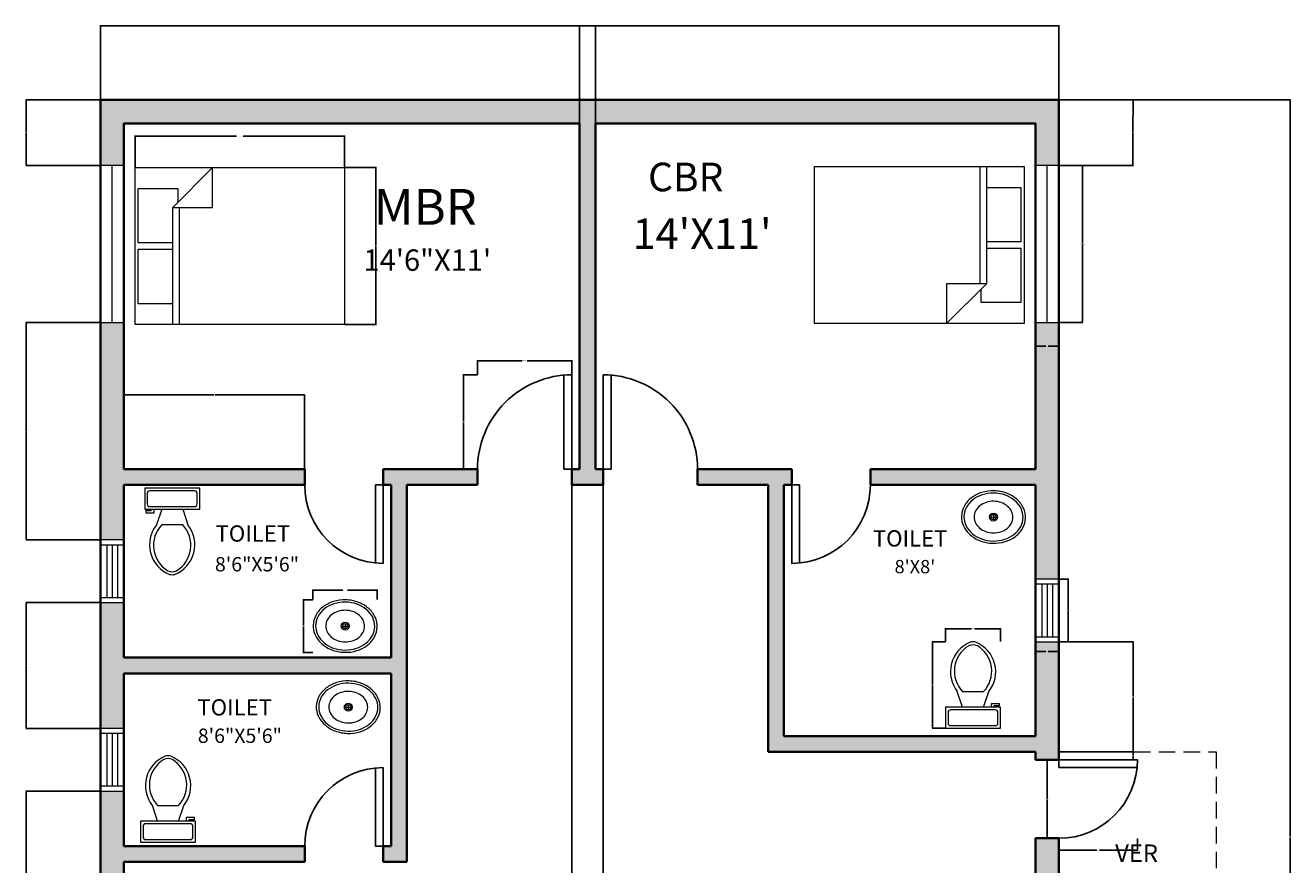
# Model space of a CAD drawing. Units: inches. Extents: x 60 to 543, y 115 to 735.
# Tile 2 of 2: x 60 to 543, y 415 to 735. Entities that reach past the tile are written whole.
import ezdxf

# ---------------------------------------------------------------- set-up
doc = ezdxf.new("R2010")
doc.units = ezdxf.units.IN
doc.linetypes.add('DASHED2', pattern=[9.525, 6.35, -3.175])
for name, color, linetype, lineweight in [('A-ANNO-DIMS', 2, 'Continuous', 18), ('A-AREA-IDEN', 7, 'Continuous', 18), ('A-DOOR', 4, 'Continuous', 25), ('A-FLOR-FIXT', 8, 'Continuous', 18), ('A-FLOR-OVHD', 8, 'DASHED2', 18), ('A-FURN', 8, 'Continuous', 18), ('A-GLAZ', 3, 'Continuous', 18), ('A-WALL', 7, 'Continuous', 35)]:
    doc.layers.add(name, color=color, linetype=linetype, lineweight=lineweight)
doc.layers.add('A-WALL-PATT', color=18, linetype='Continuous', lineweight=13, true_color=0x000000)
doc.styles.get("Standard").update_dxf_attribs({"font": 'arial.ttf'})
doc.dimstyles.get("Standard").update_dxf_attribs({"dimtxt": 0.18, "dimasz": 0.18, "dimexe": 0.18, "dimexo": 0.0625, "dimgap": 0.09, "dimtad": 0, "dimtih": 1, "dimtoh": 1, "dimdec": 4, "dimzin": 0, "dimdsep": 46, "dimtxsty": 'Standard', "dimcen": 0.09, "dimadec": 0, "dimazin": 0, "dimtfac": 1, "dimtdec": 4, "dimtofl": 0, "dimtmove": 0, "dimatfit": 3, "dimfxl": 1, "dimtolj": 1, "dimtzin": 0, "dimarcsym": 0})

# ---------------------------------------------------------------- blocks, each defined once
blk = doc.blocks.new('Bed - Queen')
for p, q in [((0, -80.00003), (0, 0)), ((0, 0), (59.99999, 0)), ((59.99999, 0), (59.99999, -80.00003)), ((7.99999, -1.2), (28.79998, -1.2)), ((7.99999, -14.4), (7.99999, -1.2)), ((28.79998, -1.2), (28.79998, -14.4)), ((31.19999, -1.2), (51.99999, -1.2)), ((31.19999, -14.4), (31.19999, -1.2)), ((51.99999, -1.2), (51.99999, -16.4)), ((0, -14.4), (44.8, -14.4)), ((59.99999, -29.6), (44.8, -14.4)), ((44.8, -14.4), (44.8, -29.6)), ((44.8, -16.8), (0, -16.8)), ((51.99999, -16.4), (46.79936, -16.4)), ((44.8, -29.6), (59.99999, -29.6)), ((59.99999, -80.00003), (0, -80.00003))]:
    blk.add_line(p, q)
blk = doc.blocks.new('Toilet - top')
for p, q in [((9.5, -6), (9.5, -2)), ((-10, -8.5), (-8, -8.5)), ((-10, -9.5), (-10, -8.5)), ((-7, -9.5), (-10, -9.5)), ((-8, -8.5), (-8, -8)), ((-7, -8), (-7, -9.5)), ((-4, -8), (-6, -14)), ((4, -8), (6, -14)), ((4, -14), (-4, -14))]:
    blk.add_line(p, q)
blk.add_lwpolyline([(10.5, -8), (10.5, 0), (-10.5, 0), (-10.5, -8)], close=True)
for points in [[(-9.5, -2), (-9.5, -6)], [(8.5, -1), (-8.5, -1)], [(-8.5, -7), (8.5, -7)]]:
    blk.add_lwpolyline(points)
for centre, radius, start, end in [((-8.62, -1.88), 0.884, 81.8699, 188.1301), ((8.62, -1.88), 0.884, 351.8699, 98.1301), ((-8.62, -6.12), 0.884, 171.8699, 278.1301), ((8.62, -6.12), 0.884, 261.8699, 8.1301), ((3.52, -21.58), 12.17, 141.4691, 247.9714), ((4.2, -21.82), 11.33, 136.3677, 238.9468), ((-3.52, -21.58), 12.17, 292.0284, 38.5307), ((-4.2, -21.82), 11.33, 301.053, 43.6321), ((0, -27.88), 4, 245.7318, 294.2682), ((0, -29), 4, 254.8605, 285.1395)]:
    blk.add_arc(centre, radius, start, end)
blk = doc.blocks.new('Sink - Oval top')
for p, q in [((-1, 0), (1, 0)), ((0, 1), (0, -1))]:
    blk.add_line(p, q)
for points in [[(-12.23, 0.39, 0.117634), (-11.46, -3.36, 0.104469), (-8.88, -6.8, 0.090016), (-5.08, -9.07, 0.08192), (-0.32, -10.02, 0.08192), (4.49, -9.38, 0.090016), (8.42, -7.36, 0.104469), (11.22, -4.09, 0.117634), (12.23, -0.39, 0.117634), (11.46, 3.36, 0.104469), (8.88, 6.8, 0.090016), (5.08, 9.07, 0.08192), (0.32, 10.02, 0.08192), (-4.49, 9.38, 0.090016), (-8.42, 7.36, 0.104469), (-11.22, 4.09, 0.117634)], [(-11.29, 0.16, 0.118622), (-10.52, -3.25, 0.104678), (-8.07, -6.36, 0.089562), (-4.54, -8.37, 0.081185), (-0.13, -9.15, 0.081185), (4.3, -8.49, 0.089562), (7.89, -6.58, 0.104678), (10.42, -3.55, 0.118622), (11.29, -0.16, 0.118622), (10.52, 3.25, 0.104678), (8.07, 6.36, 0.089562), (4.54, 8.37, 0.081185), (0.13, 9.15, 0.081185), (-4.3, 8.49, 0.089562), (-7.89, 6.58, 0.104678), (-10.42, 3.55, 0.118622)], [(-7.42, 0.08, 0.118283), (-6.91, -2.17, 0.104607), (-5.29, -4.21, 0.089718), (-2.97, -5.53, 0.081436), (-0.07, -6.04, 0.081436), (2.84, -5.59, 0.089718), (5.2, -4.33, 0.104607), (6.86, -2.32, 0.118283), (7.42, -0.08, 0.118283), (6.91, 2.17, 0.104607), (5.29, 4.21, 0.089718), (2.97, 5.53, 0.081436), (0.07, 6.04, 0.081436), (-2.84, 5.59, 0.089718), (-5.2, 4.33, 0.104607), (-6.86, 2.32, 0.118283)]]:
    blk.add_lwpolyline(points, format="xyb", close=True)
for radius in [1.5, 1]:
    blk.add_circle((0, 0), radius)
blk = doc.blocks.new('DOOR-SWING-36IN')
for p, q in [((0, 0), (0, 36)), ((0, 36), (3, 36)), ((3, 0), (3, 36))]:
    blk.add_line(p, q)
blk.add_arc((0, 36), 36, 270, 0)
blk = doc.blocks.new('DOOR-SWING-30IN')
for p, q in [((30, 30), (27, 30)), ((27, 0), (27, 30)), ((30, 0), (30, 30))]:
    blk.add_line(p, q)
blk.add_arc((30, 30), 30, 180, 270)
blk = doc.blocks.new('WINDOW-60IN')
for p, q in [((9, 60), (0, 60)), ((0, 60), (0, 0)), ((4.5, 0), (4.5, 60)), ((9, 0), (9, 60)), ((0, 0), (9, 0))]:
    blk.add_line(p, q)
blk = doc.blocks.new('BATH-VENT-24IN')
for p, q in [((0, 24), (0, 0)), ((9, 24), (0, 24)), ((9, 22), (0, 22)), ((2.5, 22), (2.5, 2)), ((4.5, 22), (4.5, 2)), ((6.5, 22), (6.5, 2)), ((9, 0), (9, 24)), ((0, 2), (9, 2)), ((0, 0), (9, 0))]:
    blk.add_line(p, q)
blk = doc.blocks.new('*D13')
at = {"layer": 'A-ANNO-DIMS', "color": 0, "lineweight": -2, "transparency": 16777216}
for p, q in [((454.43, 681.94), (463.55, 681.94)), ((463.37, 681.76), (463.37, 652.13)), ((463.37, 622.12), (463.37, 651.76)), ((454.43, 621.94), (463.55, 621.94))]:
    blk.add_line(p, q, dxfattribs=at)
at = {"layer": 'A-ANNO-DIMS', "color": 0, "transparency": 16777216}
for points in [[(463.34, 681.76), (463.4, 681.76), (463.37, 681.94)], [(463.34, 622.12), (463.4, 622.12), (463.37, 621.94)]]:
    blk.add_solid(points, dxfattribs=at)
at = {"layer": 'Defpoints', "color": 0, "transparency": 16777216}
for p in [(454.37, 681.94), (463.37, 681.94), (454.37, 621.94)]:
    blk.add_point(p, dxfattribs=at)
at = {"layer": 'A-ANNO-DIMS', "color": 0, "transparency": 16777216, "insert": (463.37, 651.94), "char_height": 0.18, "attachment_point": 5}
blk.add_mtext('\\A1;WINDOW 60 TYP.', dxfattribs=at)
blk = doc.blocks.new('*D14')
at = {"layer": 'A-ANNO-DIMS', "color": 0, "lineweight": -2, "transparency": 16777216}
for p, q in [((445.37, 621.88), (445.37, 612.76)), ((454.37, 621.88), (454.37, 612.76)), ((445.55, 612.94), (449.41, 612.94)), ((454.19, 612.94), (450.33, 612.94))]:
    blk.add_line(p, q, dxfattribs=at)
at = {"layer": 'A-ANNO-DIMS', "color": 0, "transparency": 16777216}
for points in [[(445.55, 612.97), (445.55, 612.91), (445.37, 612.94)], [(454.19, 612.97), (454.19, 612.91), (454.37, 612.94)]]:
    blk.add_solid(points, dxfattribs=at)
at = {"layer": 'Defpoints', "color": 0, "transparency": 16777216}
for p in [(445.37, 621.94), (454.37, 621.94), (454.37, 612.94)]:
    blk.add_point(p, dxfattribs=at)
at = {"layer": 'A-ANNO-DIMS', "color": 0, "transparency": 16777216, "insert": (449.87, 612.94), "char_height": 0.18, "attachment_point": 5}
blk.add_mtext('\\A1;9 TYP.', dxfattribs=at)
blk = doc.blocks.new('*D15')
at = {"layer": 'A-ANNO-DIMS', "color": 0, "lineweight": -2, "transparency": 16777216}
for p, q in [((454.33, 454.97), (449.71, 454.97)), ((449.89, 454.79), (449.89, 440.15)), ((449.89, 425.15), (449.89, 439.79)), ((454.33, 424.97), (449.71, 424.97))]:
    blk.add_line(p, q, dxfattribs=at)
at = {"layer": 'A-ANNO-DIMS', "color": 0, "transparency": 16777216}
for points in [[(449.86, 454.79), (449.92, 454.79), (449.89, 454.97)], [(449.86, 425.15), (449.92, 425.15), (449.89, 424.97)]]:
    blk.add_solid(points, dxfattribs=at)
at = {"layer": 'Defpoints', "color": 0, "transparency": 16777216}
for p in [(449.89, 454.97), (454.39, 454.97), (454.39, 424.97)]:
    blk.add_point(p, dxfattribs=at)
at = {"layer": 'A-ANNO-DIMS', "color": 0, "transparency": 16777216, "insert": (449.89, 439.97), "char_height": 0.18, "attachment_point": 5}
blk.add_mtext('\\A1;DOOR 30 TYP.', dxfattribs=at)
blk = doc.blocks.new('*D16')
at = {"layer": 'A-ANNO-DIMS', "color": 0, "lineweight": -2, "transparency": 16777216}
for p, q in [((454.39, 424.91), (454.39, 420.29)), ((454.57, 420.47), (468.87, 420.47)), ((484.21, 420.47), (469.92, 420.47)), ((484.39, 424.91), (484.39, 420.29))]:
    blk.add_line(p, q, dxfattribs=at)
at = {"layer": 'A-ANNO-DIMS', "color": 0, "transparency": 16777216}
for points in [[(454.57, 420.5), (454.57, 420.44), (454.39, 420.47)], [(484.21, 420.5), (484.21, 420.44), (484.39, 420.47)]]:
    blk.add_solid(points, dxfattribs=at)
at = {"layer": 'Defpoints', "color": 0, "transparency": 16777216}
for p in [(454.39, 424.97), (454.39, 420.47), (484.39, 424.97)]:
    blk.add_point(p, dxfattribs=at)
at = {"layer": 'A-ANNO-DIMS', "color": 0, "transparency": 16777216, "insert": (469.39, 420.47), "char_height": 0.18, "attachment_point": 5}
blk.add_mtext('\\A1;30 TYP.', dxfattribs=at)
blk = doc.blocks.new('*D17')
at = {"layer": 'A-ANNO-DIMS', "color": 0, "lineweight": -2, "transparency": 16777216}
for p, q in [((411.04, 500.05), (405.97, 500.05)), ((406.15, 499.87), (406.15, 483.71)), ((406.15, 467.18), (406.15, 483.34)), ((411.04, 467), (405.97, 467))]:
    blk.add_line(p, q, dxfattribs=at)
at = {"layer": 'A-ANNO-DIMS', "color": 0, "transparency": 16777216}
for points in [[(406.12, 499.87), (406.18, 499.87), (406.15, 500.05)], [(406.12, 467.18), (406.18, 467.18), (406.15, 467)]]:
    blk.add_solid(points, dxfattribs=at)
at = {"layer": 'Defpoints', "color": 0, "transparency": 16777216}
for p in [(411.1, 500.05), (406.15, 467), (411.1, 467)]:
    blk.add_point(p, dxfattribs=at)
at = {"layer": 'A-ANNO-DIMS', "color": 0, "transparency": 16777216, "insert": (406.15, 483.53), "char_height": 0.18, "attachment_point": 5}
blk.add_mtext('\\A1;WC 33 TYP.', dxfattribs=at)
blk = doc.blocks.new('*D18')
at = {"layer": 'A-ANNO-DIMS', "color": 0, "lineweight": -2, "transparency": 16777216}
for p, q in [((411.1, 500.11), (411.1, 505.19)), ((411.28, 505.01), (421.07, 505.01)), ((431.92, 505.01), (422.13, 505.01)), ((432.1, 500.11), (432.1, 505.19))]:
    blk.add_line(p, q, dxfattribs=at)
at = {"layer": 'A-ANNO-DIMS', "color": 0, "transparency": 16777216}
for points in [[(411.28, 505.04), (411.28, 504.98), (411.1, 505.01)], [(431.92, 505.04), (431.92, 504.98), (432.1, 505.01)]]:
    blk.add_solid(points, dxfattribs=at)
at = {"layer": 'Defpoints', "color": 0, "transparency": 16777216}
for p in [(411.1, 505.01), (411.1, 500.05), (432.1, 500.05)]:
    blk.add_point(p, dxfattribs=at)
at = {"layer": 'A-ANNO-DIMS', "color": 0, "transparency": 16777216, "insert": (421.6, 505.01), "char_height": 0.18, "attachment_point": 5}
blk.add_mtext('\\A1;21 TYP.', dxfattribs=at)
blk = doc.blocks.new('*D19')
at = {"layer": 'A-ANNO-DIMS', "color": 0, "lineweight": -2, "transparency": 16777216}
for p, q in [((169.57, 516.15), (169.57, 519.95)), ((169.75, 519.77), (180.91, 519.77)), ((193.94, 519.77), (182.78, 519.77)), ((194.12, 516.15), (194.12, 519.95))]:
    blk.add_line(p, q, dxfattribs=at)
at = {"layer": 'A-ANNO-DIMS', "color": 0, "transparency": 16777216}
for points in [[(169.75, 519.8), (169.75, 519.74), (169.57, 519.77)], [(193.94, 519.8), (193.94, 519.74), (194.12, 519.77)]]:
    blk.add_solid(points, dxfattribs=at)
at = {"layer": 'Defpoints', "color": 0, "transparency": 16777216}
for p in [(194.12, 519.77), (169.57, 516.09), (194.12, 516.09)]:
    blk.add_point(p, dxfattribs=at)
at = {"layer": 'A-ANNO-DIMS', "color": 0, "transparency": 16777216, "insert": (181.85, 519.77), "char_height": 0.18, "attachment_point": 5}
blk.add_mtext('\\A1;BASIN 25 TYP.', dxfattribs=at)
blk = doc.blocks.new('*D20')
at = {"layer": 'A-ANNO-DIMS', "color": 0, "lineweight": -2, "transparency": 16777216}
for p, q in [((169.51, 516.09), (165.71, 516.09)), ((165.89, 515.91), (165.89, 506.2)), ((165.89, 496.13), (165.89, 505.84)), ((169.51, 495.95), (165.71, 495.95))]:
    blk.add_line(p, q, dxfattribs=at)
at = {"layer": 'A-ANNO-DIMS', "color": 0, "transparency": 16777216}
for points in [[(165.86, 515.91), (165.92, 515.91), (165.89, 516.09)], [(165.86, 496.13), (165.92, 496.13), (165.89, 495.95)]]:
    blk.add_solid(points, dxfattribs=at)
at = {"layer": 'Defpoints', "color": 0, "transparency": 16777216}
for p in [(165.89, 516.09), (169.57, 516.09), (169.57, 495.95)]:
    blk.add_point(p, dxfattribs=at)
at = {"layer": 'A-ANNO-DIMS', "color": 0, "transparency": 16777216, "insert": (165.89, 506.02), "char_height": 0.18, "attachment_point": 5}
blk.add_mtext('\\A1;20 TYP.', dxfattribs=at)
blk = doc.blocks.new('*D21')
at = {"layer": 'A-ANNO-DIMS', "color": 0, "lineweight": -2, "transparency": 16777216}
for p, q in [((232.39, 602.03), (232.39, 607.55)), ((232.57, 607.37), (249.46, 607.37)), ((268.21, 607.37), (251.33, 607.37)), ((268.39, 602.03), (268.39, 607.55))]:
    blk.add_line(p, q, dxfattribs=at)
at = {"layer": 'A-ANNO-DIMS', "color": 0, "transparency": 16777216}
for points in [[(232.57, 607.4), (232.57, 607.34), (232.39, 607.37)], [(268.21, 607.4), (268.21, 607.34), (268.39, 607.37)]]:
    blk.add_solid(points, dxfattribs=at)
at = {"layer": 'Defpoints', "color": 0, "transparency": 16777216}
for p in [(232.39, 607.37), (232.39, 601.97), (268.39, 601.97)]:
    blk.add_point(p, dxfattribs=at)
at = {"layer": 'A-ANNO-DIMS', "color": 0, "transparency": 16777216, "insert": (250.39, 607.37), "char_height": 0.18, "attachment_point": 5}
blk.add_mtext('\\A1;DOOR 36 TYP.', dxfattribs=at)
blk = doc.blocks.new('*D22')
at = {"layer": 'A-ANNO-DIMS', "color": 0, "lineweight": -2, "transparency": 16777216}
for p, q in [((232.33, 601.97), (226.81, 601.97)), ((226.99, 601.79), (226.99, 584.15)), ((226.99, 566.15), (226.99, 583.79)), ((232.33, 565.97), (226.81, 565.97))]:
    blk.add_line(p, q, dxfattribs=at)
at = {"layer": 'A-ANNO-DIMS', "color": 0, "transparency": 16777216}
for points in [[(226.96, 601.79), (227.02, 601.79), (226.99, 601.97)], [(226.96, 566.15), (227.02, 566.15), (226.99, 565.97)]]:
    blk.add_solid(points, dxfattribs=at)
at = {"layer": 'Defpoints', "color": 0, "transparency": 16777216}
for p in [(232.39, 601.97), (226.99, 565.97), (232.39, 565.97)]:
    blk.add_point(p, dxfattribs=at)
at = {"layer": 'A-ANNO-DIMS', "color": 0, "transparency": 16777216, "insert": (226.99, 583.97), "char_height": 0.18, "attachment_point": 5}
blk.add_mtext('\\A1;36 TYP.', dxfattribs=at)
blk = doc.blocks.new('*D23')
at = {"layer": 'A-ANNO-DIMS', "color": 0, "lineweight": -2, "transparency": 16777216}
for p, q in [((454.46, 523.97), (458.17, 523.97)), ((457.99, 523.79), (457.99, 512.15)), ((457.99, 500.15), (457.99, 511.79)), ((454.46, 499.97), (458.17, 499.97))]:
    blk.add_line(p, q, dxfattribs=at)
at = {"layer": 'A-ANNO-DIMS', "color": 0, "transparency": 16777216}
for points in [[(457.96, 523.79), (458.02, 523.79), (457.99, 523.97)], [(457.96, 500.15), (458.02, 500.15), (457.99, 499.97)]]:
    blk.add_solid(points, dxfattribs=at)
at = {"layer": 'Defpoints', "color": 0, "transparency": 16777216}
for p in [(454.39, 523.97), (457.99, 523.97), (454.39, 499.97)]:
    blk.add_point(p, dxfattribs=at)
at = {"layer": 'A-ANNO-DIMS', "color": 0, "transparency": 16777216, "insert": (457.99, 511.97), "char_height": 0.18, "attachment_point": 5}
blk.add_mtext('\\A1;VENT 24 TYP.', dxfattribs=at)
blk = doc.blocks.new('*D24')
at = {"layer": 'A-ANNO-DIMS', "color": 0, "lineweight": -2, "transparency": 16777216}
for p, q in [((445.39, 499.91), (445.39, 496.19)), ((454.39, 499.91), (454.39, 496.19)), ((445.57, 496.37), (449.44, 496.37)), ((454.21, 496.37), (450.35, 496.37))]:
    blk.add_line(p, q, dxfattribs=at)
at = {"layer": 'A-ANNO-DIMS', "color": 0, "transparency": 16777216}
for points in [[(445.57, 496.4), (445.57, 496.34), (445.39, 496.37)], [(454.21, 496.4), (454.21, 496.34), (454.39, 496.37)]]:
    blk.add_solid(points, dxfattribs=at)
at = {"layer": 'Defpoints', "color": 0, "transparency": 16777216}
for p in [(445.39, 499.97), (454.39, 499.97), (454.39, 496.37)]:
    blk.add_point(p, dxfattribs=at)
at = {"layer": 'A-ANNO-DIMS', "color": 0, "transparency": 16777216, "insert": (449.89, 496.37), "char_height": 0.18, "attachment_point": 5}
blk.add_mtext('\\A1;9 TYP.', dxfattribs=at)
blk = doc.blocks.new('*D25')
at = {"layer": 'A-ANNO-DIMS', "color": 0, "lineweight": -2, "transparency": 16777216}
for p, q in [((101.61, 681.19), (101.61, 693.31)), ((101.79, 693.13), (140.31, 693.13)), ((181.43, 693.13), (142.91, 693.13)), ((181.61, 681.19), (181.61, 693.31))]:
    blk.add_line(p, q, dxfattribs=at)
at = {"layer": 'A-ANNO-DIMS', "color": 0, "transparency": 16777216}
for points in [[(101.79, 693.16), (101.79, 693.1), (101.61, 693.13)], [(181.43, 693.16), (181.43, 693.1), (181.61, 693.13)]]:
    blk.add_solid(points, dxfattribs=at)
at = {"layer": 'Defpoints', "color": 0, "transparency": 16777216}
for p in [(101.61, 693.13), (101.61, 681.13), (181.61, 681.13)]:
    blk.add_point(p, dxfattribs=at)
at = {"layer": 'A-ANNO-DIMS', "color": 0, "transparency": 16777216, "insert": (141.61, 693.13), "char_height": 0.18, "attachment_point": 5}
blk.add_mtext('\\A1;QUEEN BED 80 TYP.', dxfattribs=at)
blk = doc.blocks.new('*D26')
at = {"layer": 'A-ANNO-DIMS', "color": 0, "lineweight": -2, "transparency": 16777216}
for p, q in [((181.67, 681.13), (193.79, 681.13)), ((193.61, 680.95), (193.61, 651.31)), ((193.61, 621.31), (193.61, 650.95)), ((181.67, 621.13), (193.79, 621.13))]:
    blk.add_line(p, q, dxfattribs=at)
at = {"layer": 'A-ANNO-DIMS', "color": 0, "transparency": 16777216}
for points in [[(193.58, 680.95), (193.64, 680.95), (193.61, 681.13)], [(193.58, 621.31), (193.64, 621.31), (193.61, 621.13)]]:
    blk.add_solid(points, dxfattribs=at)
at = {"layer": 'Defpoints', "color": 0, "transparency": 16777216}
for p in [(181.61, 681.13), (193.61, 681.13), (181.61, 621.13)]:
    blk.add_point(p, dxfattribs=at)
at = {"layer": 'A-ANNO-DIMS', "color": 0, "transparency": 16777216, "insert": (193.61, 651.13), "char_height": 0.18, "attachment_point": 5}
blk.add_mtext('\\A1;60 TYP.', dxfattribs=at)
blk = doc.blocks.new('*D38')
at = {"layer": 'A-ANNO-DIMS', "color": 0, "lineweight": -2, "transparency": 16777216}
for p, q in [((454.46, 706.97), (542.87, 706.97)), ((542.69, 706.79), (542.69, 425.65)), ((542.69, 144.15), (542.69, 425.29)), ((454.46, 143.97), (542.87, 143.97))]:
    blk.add_line(p, q, dxfattribs=at)
at = {"layer": 'A-ANNO-DIMS', "color": 0, "transparency": 16777216}
for points in [[(542.66, 706.79), (542.72, 706.79), (542.69, 706.97)], [(542.66, 144.15), (542.72, 144.15), (542.69, 143.97)]]:
    blk.add_solid(points, dxfattribs=at)
at = {"layer": 'Defpoints', "color": 0, "transparency": 16777216}
for p in [(454.39, 706.97), (542.69, 706.97), (454.39, 143.97)]:
    blk.add_point(p, dxfattribs=at)
at = {"layer": 'A-ANNO-DIMS', "color": 0, "transparency": 16777216, "insert": (542.69, 425.47), "char_height": 0.18, "attachment_point": 5}
blk.add_mtext('\\A1;563', dxfattribs=at)
blk = doc.blocks.new('*D39')
at = {"layer": 'A-ANNO-DIMS', "color": 0, "lineweight": -2, "transparency": 16777216}
for p, q in [((88.39, 707.03), (88.39, 735.45)), ((88.57, 735.27), (271.1, 735.27)), ((454.21, 735.27), (271.68, 735.27)), ((454.39, 707.03), (454.39, 735.45))]:
    blk.add_line(p, q, dxfattribs=at)
at = {"layer": 'A-ANNO-DIMS', "color": 0, "transparency": 16777216}
for points in [[(88.57, 735.3), (88.57, 735.24), (88.39, 735.27)], [(454.21, 735.3), (454.21, 735.24), (454.39, 735.27)]]:
    blk.add_solid(points, dxfattribs=at)
at = {"layer": 'Defpoints', "color": 0, "transparency": 16777216}
for p in [(454.39, 735.27), (88.39, 706.97), (454.39, 706.97)]:
    blk.add_point(p, dxfattribs=at)
at = {"layer": 'A-ANNO-DIMS', "color": 0, "transparency": 16777216, "insert": (271.39, 735.27), "char_height": 0.18, "attachment_point": 5}
blk.add_mtext('\\A1;366', dxfattribs=at)
blk = doc.blocks.new('*D42')
at = {"layer": 'A-ANNO-DIMS', "color": 0, "lineweight": -2, "transparency": 16777216}
for p, q in [((88.33, 442.97), (59.91, 442.97)), ((60.09, 442.79), (60.09, 401.54)), ((60.09, 359.92), (60.09, 401.17)), ((88.33, 359.74), (59.91, 359.74))]:
    blk.add_line(p, q, dxfattribs=at)
at = {"layer": 'A-ANNO-DIMS', "color": 0, "transparency": 16777216}
for points in [[(60.06, 442.79), (60.12, 442.79), (60.09, 442.97)], [(60.06, 359.92), (60.12, 359.92), (60.09, 359.74)]]:
    blk.add_solid(points, dxfattribs=at)
at = {"layer": 'Defpoints', "color": 0, "transparency": 16777216}
for p in [(60.09, 442.97), (88.39, 442.97), (88.39, 359.74)]:
    blk.add_point(p, dxfattribs=at)
at = {"layer": 'A-ANNO-DIMS', "color": 0, "transparency": 16777216, "insert": (60.09, 401.35), "char_height": 0.18, "attachment_point": 5}
blk.add_mtext('\\A1;83.23', dxfattribs=at)
blk = doc.blocks.new('*D43')
at = {"layer": 'A-ANNO-DIMS', "color": 0, "lineweight": -2, "transparency": 16777216}
for p, q in [((88.33, 514.97), (59.91, 514.97)), ((60.09, 514.79), (60.09, 491.15)), ((60.09, 467.15), (60.09, 490.79)), ((88.33, 466.97), (59.91, 466.97))]:
    blk.add_line(p, q, dxfattribs=at)
at = {"layer": 'A-ANNO-DIMS', "color": 0, "transparency": 16777216}
for points in [[(60.06, 514.79), (60.12, 514.79), (60.09, 514.97)], [(60.06, 467.15), (60.12, 467.15), (60.09, 466.97)]]:
    blk.add_solid(points, dxfattribs=at)
at = {"layer": 'Defpoints', "color": 0, "transparency": 16777216}
for p in [(60.09, 514.97), (88.39, 514.97), (88.39, 466.97)]:
    blk.add_point(p, dxfattribs=at)
at = {"layer": 'A-ANNO-DIMS', "color": 0, "transparency": 16777216, "insert": (60.09, 490.97), "char_height": 0.18, "attachment_point": 5}
blk.add_mtext('\\A1;48', dxfattribs=at)
blk = doc.blocks.new('*D44')
at = {"layer": 'A-ANNO-DIMS', "color": 0, "lineweight": -2, "transparency": 16777216}
for p, q in [((88.33, 621.95), (59.91, 621.95)), ((60.09, 621.77), (60.09, 580.64)), ((60.09, 539.15), (60.09, 580.28)), ((88.33, 538.97), (59.91, 538.97))]:
    blk.add_line(p, q, dxfattribs=at)
at = {"layer": 'A-ANNO-DIMS', "color": 0, "transparency": 16777216}
for points in [[(60.06, 621.77), (60.12, 621.77), (60.09, 621.95)], [(60.06, 539.15), (60.12, 539.15), (60.09, 538.97)]]:
    blk.add_solid(points, dxfattribs=at)
at = {"layer": 'Defpoints', "color": 0, "transparency": 16777216}
for p in [(60.09, 621.95), (88.39, 621.95), (88.39, 538.97)]:
    blk.add_point(p, dxfattribs=at)
at = {"layer": 'A-ANNO-DIMS', "color": 0, "transparency": 16777216, "insert": (60.09, 580.46), "char_height": 0.18, "attachment_point": 5}
blk.add_mtext('\\A1;82.98', dxfattribs=at)
blk = doc.blocks.new('*D45')
at = {"layer": 'A-ANNO-DIMS', "color": 0, "lineweight": -2, "transparency": 16777216}
for p, q in [((88.33, 706.97), (59.91, 706.97)), ((60.09, 706.79), (60.09, 694.64)), ((60.09, 682.13), (60.09, 694.28)), ((88.33, 681.95), (59.91, 681.95))]:
    blk.add_line(p, q, dxfattribs=at)
at = {"layer": 'A-ANNO-DIMS', "color": 0, "transparency": 16777216}
for points in [[(60.06, 706.79), (60.12, 706.79), (60.09, 706.97)], [(60.06, 682.13), (60.12, 682.13), (60.09, 681.95)]]:
    blk.add_solid(points, dxfattribs=at)
at = {"layer": 'Defpoints', "color": 0, "transparency": 16777216}
for p in [(60.09, 706.97), (88.39, 706.97), (88.39, 681.95)]:
    blk.add_point(p, dxfattribs=at)
at = {"layer": 'A-ANNO-DIMS', "color": 0, "transparency": 16777216, "insert": (60.09, 694.46), "char_height": 0.18, "attachment_point": 5}
blk.add_mtext('\\A1;25.024', dxfattribs=at)
blk = doc.blocks.new('*D47')
at = {"layer": 'A-ANNO-DIMS', "color": 0, "lineweight": -2, "transparency": 16777216}
for p, q in [((454.46, 457.97), (482.87, 457.97)), ((454.46, 454.97), (482.87, 454.97)), ((482.69, 457.79), (482.69, 456.65)), ((482.69, 455.15), (482.69, 456.29))]:
    blk.add_line(p, q, dxfattribs=at)
at = {"layer": 'A-ANNO-DIMS', "color": 0, "transparency": 16777216}
for points in [[(482.66, 457.79), (482.72, 457.79), (482.69, 457.97)], [(482.66, 455.15), (482.72, 455.15), (482.69, 454.97)]]:
    blk.add_solid(points, dxfattribs=at)
at = {"layer": 'Defpoints', "color": 0, "transparency": 16777216}
for p in [(454.39, 457.97), (454.39, 454.97), (482.69, 454.97)]:
    blk.add_point(p, dxfattribs=at)
at = {"layer": 'A-ANNO-DIMS', "color": 0, "transparency": 16777216, "insert": (482.69, 456.47), "char_height": 0.18, "attachment_point": 5}
blk.add_mtext('\\A1;3', dxfattribs=at)
blk = doc.blocks.new('*D48')
at = {"layer": 'A-ANNO-DIMS', "color": 0, "lineweight": -2, "transparency": 16777216}
for p, q in [((454.46, 499.97), (482.87, 499.97)), ((482.69, 499.79), (482.69, 479.15)), ((482.69, 458.15), (482.69, 478.79)), ((454.46, 457.97), (482.87, 457.97))]:
    blk.add_line(p, q, dxfattribs=at)
at = {"layer": 'A-ANNO-DIMS', "color": 0, "transparency": 16777216}
for points in [[(482.66, 499.79), (482.72, 499.79), (482.69, 499.97)], [(482.66, 458.15), (482.72, 458.15), (482.69, 457.97)]]:
    blk.add_solid(points, dxfattribs=at)
at = {"layer": 'Defpoints', "color": 0, "transparency": 16777216}
for p in [(454.39, 499.97), (454.39, 457.97), (482.69, 457.97)]:
    blk.add_point(p, dxfattribs=at)
at = {"layer": 'A-ANNO-DIMS', "color": 0, "transparency": 16777216, "insert": (482.69, 478.97), "char_height": 0.18, "attachment_point": 5}
blk.add_mtext('\\A1;42', dxfattribs=at)
blk = doc.blocks.new('*D49')
at = {"layer": 'A-ANNO-DIMS', "color": 0, "lineweight": -2, "transparency": 16777216}
for p, q in [((454.46, 706.97), (482.87, 706.94)), ((482.69, 706.76), (482.68, 694.61)), ((482.67, 682.1), (482.68, 694.25)), ((454.43, 681.94), (482.85, 681.92))]:
    blk.add_line(p, q, dxfattribs=at)
at = {"layer": 'A-ANNO-DIMS', "color": 0, "transparency": 16777216}
for points in [[(482.66, 706.76), (482.72, 706.76), (482.69, 706.94)], [(482.64, 682.1), (482.7, 682.1), (482.67, 681.92)]]:
    blk.add_solid(points, dxfattribs=at)
at = {"layer": 'Defpoints', "color": 0, "transparency": 16777216}
for p in [(454.39, 706.97), (454.37, 681.94), (482.67, 681.92)]:
    blk.add_point(p, dxfattribs=at)
at = {"layer": 'A-ANNO-DIMS', "color": 0, "transparency": 16777216, "insert": (482.68, 694.43), "char_height": 0.18, "attachment_point": 5}
blk.add_mtext('\\A1;25.024', dxfattribs=at)
blk = doc.blocks.new('*D51')
at = {"layer": 'A-ANNO-DIMS', "color": 0, "lineweight": -2, "transparency": 16777216}
for p, q in [((271.39, 698.03), (271.39, 735.45)), ((271.57, 735.27), (274.24, 735.27)), ((277.21, 735.27), (274.54, 735.27)), ((277.39, 698.03), (277.39, 735.45))]:
    blk.add_line(p, q, dxfattribs=at)
at = {"layer": 'A-ANNO-DIMS', "color": 0, "transparency": 16777216}
for points in [[(271.57, 735.3), (271.57, 735.24), (271.39, 735.27)], [(277.21, 735.3), (277.21, 735.24), (277.39, 735.27)]]:
    blk.add_solid(points, dxfattribs=at)
at = {"layer": 'Defpoints', "color": 0, "transparency": 16777216}
for p in [(277.39, 735.27), (271.39, 697.97), (277.39, 697.97)]:
    blk.add_point(p, dxfattribs=at)
at = {"layer": 'A-ANNO-DIMS', "color": 0, "transparency": 16777216, "insert": (274.39, 735.27), "char_height": 0.18, "attachment_point": 5}
blk.add_mtext('\\A1;6', dxfattribs=at)
blk = doc.blocks.new('*D55')
at = {"layer": 'A-ANNO-DIMS', "color": 0, "lineweight": -2, "transparency": 16777216}
for p, q in [((268.39, 559.91), (268.39, 115.49)), ((280.39, 559.91), (280.39, 115.49)), ((268.57, 115.67), (274.18, 115.67)), ((280.21, 115.67), (274.6, 115.67))]:
    blk.add_line(p, q, dxfattribs=at)
at = {"layer": 'A-ANNO-DIMS', "color": 0, "transparency": 16777216}
for points in [[(268.57, 115.7), (268.57, 115.64), (268.39, 115.67)], [(280.21, 115.7), (280.21, 115.64), (280.39, 115.67)]]:
    blk.add_solid(points, dxfattribs=at)
at = {"layer": 'Defpoints', "color": 0, "transparency": 16777216}
for p in [(268.39, 559.97), (280.39, 559.97), (280.39, 115.67)]:
    blk.add_point(p, dxfattribs=at)
at = {"layer": 'A-ANNO-DIMS', "color": 0, "transparency": 16777216, "insert": (274.39, 115.67), "char_height": 0.18, "attachment_point": 5}
blk.add_mtext('\\A1;12', dxfattribs=at)
blk = doc.blocks.new('*D56')
at = {"layer": 'A-ANNO-DIMS', "color": 0, "lineweight": -2, "transparency": 16777216}
for p, q in [((97.39, 566.03), (97.39, 594.45)), ((166.39, 566.03), (166.39, 594.45)), ((97.57, 594.27), (131.67, 594.27)), ((166.21, 594.27), (132.11, 594.27))]:
    blk.add_line(p, q, dxfattribs=at)
at = {"layer": 'A-ANNO-DIMS', "color": 0, "transparency": 16777216}
for points in [[(97.57, 594.3), (97.57, 594.24), (97.39, 594.27)], [(166.21, 594.3), (166.21, 594.24), (166.39, 594.27)]]:
    blk.add_solid(points, dxfattribs=at)
at = {"layer": 'Defpoints', "color": 0, "transparency": 16777216}
for p in [(166.39, 594.27), (97.39, 565.97), (166.39, 565.97)]:
    blk.add_point(p, dxfattribs=at)
at = {"layer": 'A-ANNO-DIMS', "color": 0, "transparency": 16777216, "insert": (131.89, 594.27), "char_height": 0.18, "attachment_point": 5}
blk.add_mtext('\\A1;69', dxfattribs=at)

msp = doc.modelspace()

# ---------------------------------------------------------------- hatches: boundary and pattern name
at = {"layer": 'A-WALL-PATT'}
h = msp.add_hatch(color=256, dxfattribs=at)
h.dxf.hatch_style = 1
h.paths.add_polyline_path([(454.3937, 706.9693), (277.3937, 706.9693), (271.3937, 706.9693), (88.3937, 706.9693), (88.3937, 681.945), (97.3937, 681.945), (97.3937, 697.9693), (271.3937, 697.9693), (271.3937, 565.9693), (268.3937, 565.9693), (268.3937, 559.9693), (271.3937, 559.9693), (277.3937, 559.9693), (280.3937, 559.9693), (280.3937, 565.9693), (277.3937, 565.9693), (277.3937, 697.9693), (445.3937, 697.9693), (445.3937, 681.945), (454.3937, 681.945)])
h.paths.add_polyline_path([(97.3937, 621.945), (88.3937, 621.945), (88.3937, 565.9693), (88.3937, 538.9693), (97.3937, 538.9693), (97.3937, 559.9693), (166.3937, 559.9693), (166.3937, 565.9693), (97.3937, 565.9693)])
h.paths.add_polyline_path([(454.3937, 621.945), (445.3937, 621.945), (445.3937, 565.9693), (382.3937, 565.9693), (382.3937, 559.9693), (445.3937, 559.9693), (445.3937, 523.9693), (454.3937, 523.9693), (454.3937, 559.9693), (454.3937, 565.9693)])
h.paths.add_polyline_path([(352.3937, 565.9693), (316.3937, 565.9693), (316.3937, 559.9693), (343.3937, 559.9693), (343.3937, 457.9693), (445.3937, 457.9693), (445.3937, 454.9693), (454.3937, 454.9693), (454.3937, 499.9693), (445.3937, 499.9693), (445.3937, 463.9693), (349.3937, 463.9693), (349.3937, 559.9693), (352.3937, 559.9693)])
h.paths.add_polyline_path([(232.3937, 565.9693), (196.3937, 565.9693), (196.3937, 559.9693), (199.3937, 559.9693), (199.3937, 493.9693), (97.3937, 493.9693), (97.3937, 514.9693), (88.3937, 514.9693), (88.3937, 466.9693), (97.3937, 466.9693), (97.3937, 487.9693), (199.3937, 487.9693), (199.3937, 421.9693), (196.3937, 421.9693), (196.3937, 415.9693), (199.3937, 415.9693), (205.3937, 415.9693), (205.3937, 421.9693), (205.3937, 493.9693), (205.3937, 559.9693), (232.3937, 559.9693)])
h.paths.add_polyline_path([(97.3937, 415.9693), (166.3937, 415.9693), (166.3937, 421.9693), (97.3937, 421.9693), (97.3937, 442.9693), (88.3937, 442.9693), (88.3937, 421.9693), (88.3937, 359.7372), (97.3937, 359.7372)])
h.paths.add_polyline_path([(97.3937, 299.7372), (88.3937, 299.7372), (88.3937, 225.2372), (97.3937, 225.2372), (97.3937, 236.9693), (199.3937, 236.9693), (268.3937, 236.9693), (268.3937, 242.9693), (199.3937, 242.9693), (97.3937, 242.9693)])
h.paths.add_polyline_path([(97.3937, 165.2372), (88.3937, 165.2372), (88.3937, 143.9693), (97.3937, 143.9693), (199.3937, 143.9693), (325.3937, 143.9693), (325.3937, 164.9693), (319.3937, 164.9693), (319.3937, 152.9693), (199.3937, 152.9693), (97.3937, 152.9693)])
h.paths.add_polyline_path([(454.3937, 242.9693), (454.3937, 278.9693), (445.3937, 278.9693), (445.3937, 242.9693), (325.3937, 242.9693), (325.3937, 374.9693), (328.3937, 374.9693), (328.3937, 380.9693), (319.3937, 380.9693), (319.3937, 242.9693), (316.3937, 242.9693), (316.3937, 236.9693), (319.3937, 236.9693), (319.3937, 222.9693), (325.3937, 222.9693), (325.3937, 236.9693), (454.3937, 236.9693)])
h.paths.add_polyline_path([(454.3937, 424.9693), (445.3937, 424.9693), (445.3937, 380.9693), (364.3937, 380.9693), (364.3937, 374.9693), (445.3937, 374.9693), (445.3937, 338.9693), (454.3937, 338.9693), (454.3937, 346.9693)])

# ---------------------------------------------------------------- linework, layer by layer
at = {"layer": 'A-FLOR-OVHD'}
for p, q in [((454.3937, 457.9693), (514.3937, 457.9693)), ((514.3937, 457.9693), (514.3937, 346.9693)), ((454.3937, 424.9693), (454.3937, 346.9693))]:
    msp.add_line(p, q, dxfattribs=at)
at = {"layer": 'A-WALL'}
for p, q in [((271.3937, 706.9693), (277.3937, 706.9693)), ((277.3937, 706.9693), (445.3937, 706.9693)), ((271.3937, 565.9693), (271.3937, 697.9693)), ((277.3937, 565.9693), (277.3937, 697.9693)), ((454.3937, 565.9693), (454.3937, 697.9693)), ((88.3937, 565.9693), (88.3937, 421.9693)), ((97.3937, 565.9693), (166.3937, 565.9693)), ((166.3937, 565.9693), (97.3937, 565.9693)), ((166.3937, 559.9693), (166.3937, 565.9693)), ((199.3937, 565.9693), (196.3937, 565.9693)), ((196.3937, 559.9693), (196.3937, 565.9693)), ((196.3937, 565.9693), (232.3937, 565.9693)), ((232.3937, 565.9693), (232.3937, 559.9693)), ((268.3937, 565.9693), (268.3937, 559.9693)), ((268.3937, 565.9693), (271.3937, 565.9693)), ((280.3937, 565.9693), (277.3937, 565.9693)), ((280.3937, 565.9693), (280.3937, 559.9693)), ((316.3937, 565.9693), (316.3937, 559.9693)), ((352.3937, 565.9693), (316.3937, 565.9693)), ((352.3937, 565.9693), (352.3937, 559.9693)), ((445.3937, 565.9693), (382.3937, 565.9693)), ((382.3937, 565.9693), (382.3937, 559.9693)), ((454.3937, 565.9693), (454.3937, 559.9693)), ((97.3937, 559.9693), (97.3937, 493.9693)), ((97.3937, 559.9693), (166.3937, 559.9693)), ((196.3937, 559.9693), (199.3937, 559.9693)), ((199.3937, 493.9693), (199.3937, 559.9693)), ((205.3937, 493.9693), (205.3937, 559.9693)), ((205.3937, 559.9693), (232.3937, 559.9693)), ((268.3937, 559.9693), (271.3937, 559.9693)), ((271.3937, 559.9693), (277.3937, 559.9693)), ((277.3937, 559.9693), (280.3937, 559.9693)), ((280.3937, 559.9693), (277.3937, 559.9693)), ((316.3937, 559.9693), (343.3937, 559.9693)), ((343.3937, 559.9693), (316.3937, 559.9693)), ((343.3937, 559.9693), (343.3937, 457.9693)), ((349.3937, 559.9693), (349.3937, 463.9693)), ((352.3937, 559.9693), (349.3937, 559.9693)), ((349.3937, 559.9693), (352.3937, 559.9693)), ((445.3937, 559.9693), (382.3937, 559.9693)), ((382.3937, 559.9693), (445.3937, 559.9693)), ((445.3937, 559.9693), (445.3937, 463.9693)), ((454.3937, 559.9693), (454.3937, 454.9693)), ((97.3937, 493.9693), (199.3937, 493.9693)), ((205.3937, 421.9693), (205.3937, 493.9693)), ((97.3937, 487.9693), (199.3937, 487.9693)), ((97.3937, 487.9693), (97.3937, 421.9693)), ((199.3937, 421.9693), (199.3937, 487.9693)), ((349.3937, 463.9693), (445.3937, 463.9693)), ((343.3937, 457.9693), (445.3937, 457.9693)), ((445.3937, 457.9693), (445.3937, 454.9693)), ((445.3937, 454.9693), (454.3937, 454.9693)), ((88.3937, 421.9693), (88.3937, 143.9693)), ((97.3937, 421.9693), (166.3937, 421.9693)), ((166.3937, 421.9693), (166.3937, 415.9693)), ((196.3937, 421.9693), (196.3937, 415.9693)), ((196.3937, 421.9693), (199.3937, 421.9693)), ((205.3937, 421.9693), (205.3937, 415.9693)), ((445.3937, 424.9693), (454.3937, 424.9693)), ((445.3937, 424.9693), (445.3937, 380.9693)), ((454.3937, 424.9693), (454.3937, 346.9693)), ((97.3937, 415.9693), (166.3937, 415.9693)), ((97.3937, 415.9693), (97.3937, 242.9693)), ((196.3937, 415.9693), (199.3937, 415.9693)), ((199.3937, 415.9693), (205.3937, 415.9693))]:
    msp.add_line(p, q, dxfattribs=at)
for points in [[(271.3937, 706.9693), (88.3937, 706.9693), (88.3937, 565.9693)], [(277.3937, 706.9693), (454.3937, 706.9693), (454.3937, 565.9693)], [(271.3937, 697.9693), (97.3937, 697.9693), (97.3937, 565.9693)], [(277.3937, 697.9693), (445.3937, 697.9693), (445.3937, 565.9693)]]:
    msp.add_lwpolyline(points, dxfattribs=at)

# ---------------------------------------------------------------- block references
at = {"layer": 'A-DOOR'}
for name, p, rotation in [('DOOR-SWING-36IN', (268.3934, 601.9697), 180), ('DOOR-SWING-30IN', (484.394, 424.9696), 89.99999999999982)]:
    msp.add_blockref(name, p, dxfattribs=dict(at, rotation=rotation))
at = {"layer": 'A-DOOR', "extrusion": (0, 0, -1), "zscale": -1, "rotation": 180}
for name, p in [('DOOR-SWING-36IN', (-280.394, 601.9697)), ('DOOR-SWING-30IN', (-166.394, 451.9697))]:
    msp.add_blockref(name, p, dxfattribs=at)
at = {"layer": 'A-DOOR'}
msp.add_blockref('DOOR-SWING-30IN', (166.394, 529.969), dxfattribs=at)
at = {"layer": 'A-DOOR', "extrusion": (0, 0, -1), "zscale": -1}
msp.add_blockref('DOOR-SWING-30IN', (-382.3934, 529.969), dxfattribs=at)
at = {"layer": 'A-FLOR-FIXT'}
for name, p in [('Toilet - top', (115.8071, 558.6387)), ('Sink - Oval top', (429.4058, 547.6501)), ('Sink - Oval top', (181.8476, 506.0185)), ('Sink - Oval top', (183.0426, 475.0569))]:
    msp.add_blockref(name, p, dxfattribs=at)
at = {"layer": 'A-FLOR-FIXT', "rotation": 180}
for p in [(421.6026, 467.0033), (114.223, 423.5107)]:
    msp.add_blockref('Toilet - top', p, dxfattribs=at)
at = {"layer": 'A-FURN'}
for p, rotation in [((441.0847, 681.5342), 270), ((101.6102, 621.1298), 90)]:
    msp.add_blockref('Bed - Queen', p, dxfattribs=dict(at, rotation=rotation))
at = {"layer": 'A-GLAZ'}
for name, p in [('WINDOW-60IN', (88.394, 621.945)), ('WINDOW-60IN', (445.3694, 621.945)), ('BATH-VENT-24IN', (88.394, 514.969)), ('BATH-VENT-24IN', (445.394, 499.969)), ('BATH-VENT-24IN', (88.394, 442.969))]:
    msp.add_blockref(name, p, dxfattribs=at)

# ---------------------------------------------------------------- texts
at = {"layer": 'A-AREA-IDEN', "attachment_point": 1}
for s, width, gutter_width, insert, char_height in [('CBR', 539.060824, 54.6236, (297.5084, 682.992), 10.92473), ('MBR', 676.236228, 68.5238, (192.7899, 672.9576), 13.70475), ("14'X11'", 573.206074, 58.0836, (291.6013, 661.6749), 11.61672), ('14\'6"X11\'', 402.899641, 40.8263, (188.8379, 649.8564), 8.16525), ('TOILET', 305.990582, 31.0064, (132.3623, 544.4751), 6.20127), ('TOILET', 305.990582, 31.0064, (383.3481, 542.6099), 6.20127), ('8\'6"X5\'6"', 270.169123, 27.3765, (132.1332, 532.3694), 5.47531), ("8'X8'", 250.819135, 25.4158, (391.648, 531.2672), 5.08316), ('TOILET', 305.990582, 31.0064, (125.4363, 478.0801), 6.20127), ('8\'6"X5\'6"', 270.169123, 27.3765, (125.5926, 466.8824), 5.47531), ('VER', 328.793513, 33.317, (475.8743, 422.6351), 6.6634)]:
    msp.add_mtext_dynamic_manual_height_columns(s, width=width, gutter_width=gutter_width, heights=[0], dxfattribs=dict(at, insert=insert, char_height=char_height))

# ---------------------------------------------------------------- dimensions: what is measured, and where the dimension line sits
at = {"layer": 'A-ANNO-DIMS'}
for base, p1, p2, picture, middle in [((454.3937, 735.2693), (88.3937, 706.9693), (454.3937, 706.9693), '*D39', (271.3937, 735.2693)), ((277.3937, 735.2693), (271.3937, 697.9693), (277.3937, 697.9693), '*D51', (274.3937, 735.2693)), ((166.3937, 594.2693), (97.3937, 565.9693), (166.3937, 565.9693), '*D56', (131.8937, 594.2693)), ((280.3937, 115.6693), (268.3937, 559.9693), (280.3937, 559.9693), '*D55', (274.3937, 115.6693))]:
    dim = msp.add_linear_dim(base=base, p1=p1, p2=p2, dimstyle='Standard', override={"dimdec": 0, "dimlfac": 1, "dimrnd": 0, "dimzin": 0, "dimdsep": 46, "dimlunit": 2}, dxfattribs=at)
    dim.commit()
    dim.dimension.update_dxf_attribs({"geometry": picture, "text_midpoint": middle})
for base, p1, p2, angle, override, picture, middle in [((60.0937, 706.9693), (88.3937, 681.945), (88.3937, 706.9693), 90, {"dimdec": 3, "dimlfac": 1, "dimrnd": 0, "dimzin": 0, "dimdsep": 46, "dimlunit": 2}, '*D45', (60.0937, 694.4572)), ((482.6691, 681.9172), (454.3937, 706.9693), (454.3691, 681.945), 269.94362, {"dimdec": 3, "dimlfac": 1, "dimrnd": 0, "dimzin": 0, "dimdsep": 46, "dimlunit": 2}, '*D49', (482.6814, 694.4293)), ((542.6937, 706.9693), (454.3937, 143.9693), (454.3937, 706.9693), 90, {"dimdec": 0, "dimlfac": 1, "dimrnd": 0, "dimzin": 0, "dimdsep": 46, "dimlunit": 2}, '*D38', (542.6937, 425.4693)), ((60.0937, 621.945), (88.3937, 538.9693), (88.3937, 621.945), 90, {"dimdec": 2, "dimlfac": 1, "dimrnd": 0, "dimzin": 0, "dimdsep": 46, "dimlunit": 2}, '*D44', (60.0937, 580.4572)), ((60.0937, 514.9693), (88.3937, 466.9693), (88.3937, 514.9693), 90, {"dimdec": 0, "dimlfac": 1, "dimrnd": 0, "dimzin": 0, "dimdsep": 46, "dimlunit": 2}, '*D43', (60.0937, 490.9693)), ((482.6937, 457.9693), (454.3937, 499.9693), (454.3937, 457.9693), 270, {"dimdec": 0, "dimlfac": 1, "dimrnd": 0, "dimzin": 0, "dimdsep": 46, "dimlunit": 2}, '*D48', (482.6937, 478.9693)), ((482.6937, 454.9693), (454.3937, 457.9693), (454.3937, 454.9693), 270, {"dimdec": 0, "dimlfac": 1, "dimrnd": 0, "dimzin": 0, "dimdsep": 46, "dimlunit": 2}, '*D47', (482.6937, 456.4693)), ((60.0937, 442.9693), (88.3937, 359.7372), (88.3937, 442.9693), 90, {"dimdec": 2, "dimlfac": 1, "dimrnd": 0, "dimzin": 0, "dimdsep": 46, "dimlunit": 2}, '*D42', (60.0937, 401.3533))]:
    dim = msp.add_linear_dim(base=base, p1=p1, p2=p2, angle=angle, dimstyle='Standard', override=override, dxfattribs=at)
    dim.commit()
    dim.dimension.update_dxf_attribs({"geometry": picture, "text_midpoint": middle})
for base, p1, p2, angle, text, picture, middle in [((101.6102, 693.1298), (181.6103, 681.1298), (101.6102, 681.1298), 180, 'QUEEN BED <> TYP.', '*D25', (141.6103, 693.1298)), ((463.3691, 681.945), (454.3691, 621.945), (454.3691, 681.945), 90, 'WINDOW <> TYP.', '*D13', (463.3691, 651.945)), ((193.6103, 681.1298), (181.6103, 621.1298), (181.6103, 681.1298), 90, '<> TYP.', '*D26', (193.6103, 651.1298)), ((232.3937, 607.3693), (268.3937, 601.9693), (232.3937, 601.9693), 180, 'DOOR <> TYP.', '*D21', (250.3937, 607.3693)), ((226.9937, 565.9693), (232.3937, 601.9693), (232.3937, 565.9693), 270, '<> TYP.', '*D22', (226.9937, 583.9693)), ((457.9937, 523.9693), (454.3937, 499.9693), (454.3937, 523.9693), 90, 'VENT <> TYP.', '*D23', (457.9937, 511.9693)), ((165.8895, 516.0868), (169.5721, 495.9502), (169.5721, 516.0868), 90, '<> TYP.', '*D20', (165.8895, 506.0185)), ((411.1026, 505.0064), (432.1026, 500.0495), (411.1026, 500.0495), 180, '<> TYP.', '*D18', (421.6026, 505.0064)), ((406.1457, 467.0033), (411.1026, 500.0495), (411.1026, 467.0033), 270, 'WC <> TYP.', '*D17', (406.1457, 483.5264)), ((449.8937, 454.9693), (454.3937, 424.9693), (454.3937, 454.9693), 90, 'DOOR <> TYP.', '*D15', (449.8937, 439.9693)), ((454.3937, 420.4693), (484.3937, 424.9693), (454.3937, 424.9693), 180, '<> TYP.', '*D16', (469.3937, 420.4693))]:
    dim = msp.add_linear_dim(base=base, p1=p1, p2=p2, angle=angle, text=text, dimstyle='Standard', override={"dimdec": 0, "dimlfac": 1, "dimrnd": 0, "dimzin": 0, "dimdsep": 46, "dimlunit": 2}, dxfattribs=at)
    dim.commit()
    dim.dimension.update_dxf_attribs({"geometry": picture, "text_midpoint": middle})
for base, p1, p2, text, picture, middle in [((454.3691, 612.945), (445.3691, 621.945), (454.3691, 621.945), '<> TYP.', '*D14', (449.8691, 612.945)), ((194.123, 519.7695), (169.5721, 516.0868), (194.123, 516.0868), 'BASIN <> TYP.', '*D19', (181.8476, 519.7695)), ((454.3937, 496.3693), (445.3937, 499.9693), (454.3937, 499.9693), '<> TYP.', '*D24', (449.8937, 496.3693))]:
    dim = msp.add_linear_dim(base=base, p1=p1, p2=p2, text=text, dimstyle='Standard', override={"dimdec": 0, "dimlfac": 1, "dimrnd": 0, "dimzin": 0, "dimdsep": 46, "dimlunit": 2}, dxfattribs=at)
    dim.commit()
    dim.dimension.update_dxf_attribs({"geometry": picture, "text_midpoint": middle})

doc.saveas('drawing.dxf')
